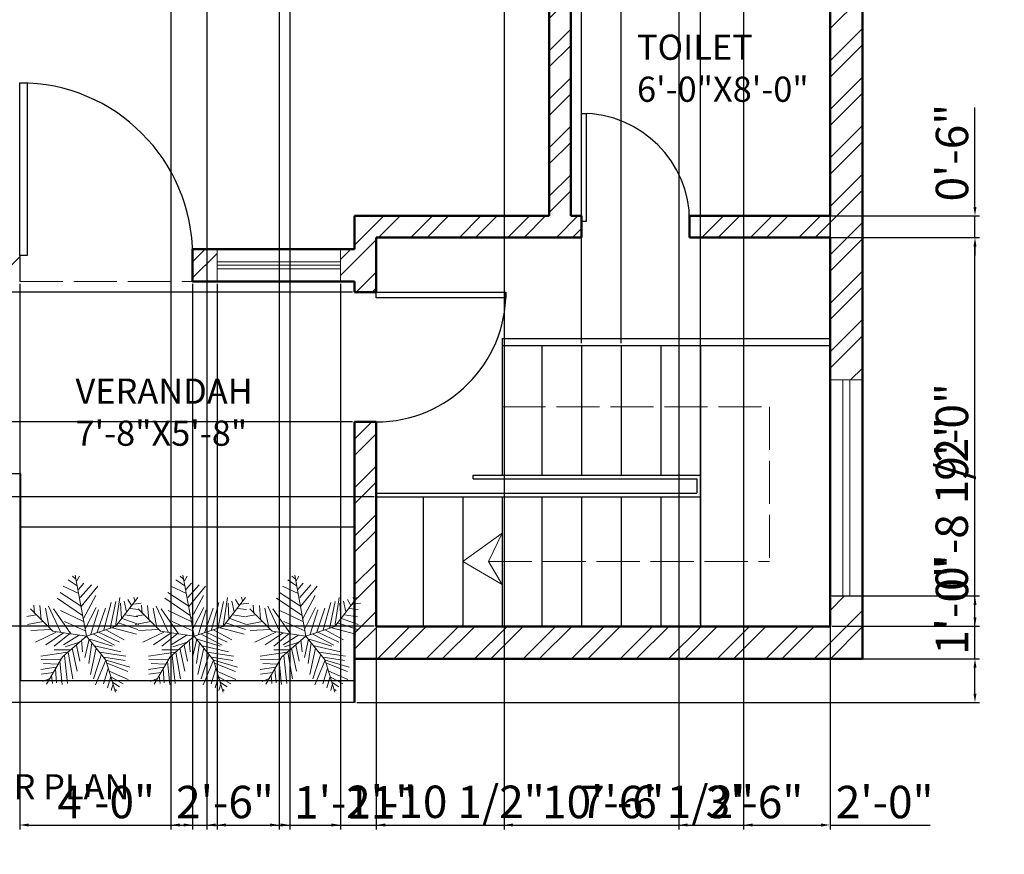
# Model space of a CAD drawing. Units: inches. Extents: x 1104 to 1745, y 678 to 1361.
# Tile 2 of 4: x 1387 to 1660, y 678 to 910. Entities that reach past the tile are written whole.
import ezdxf

# ---------------------------------------------------------------- set-up
doc = ezdxf.new("R2010")
doc.units = ezdxf.units.IN
doc.linetypes.add('ACAD_ISO02W100', pattern=[15, 12, -3])
for name, color, linetype, lineweight in [('A-ANNO-DIMS', 2, 'Continuous', 18), ('A-ANNO-PATH', 2, 'ACAD_ISO02W100', 18), ('A-ANNO-SYMB', 2, 'Continuous', 18), ('A-ANNO-TEXT', 7, 'Continuous', 35), ('A-AREA-IDEN', 7, 'Continuous', 25), ('A-DOOR', 4, 'Continuous', 25), ('A-DOOR-HIDN', 4, 'ACAD_ISO02W100', 18), ('A-FLOR-STRS', 7, 'Continuous', 25), ('A-WALL', 7, 'Continuous', 50), ('A-WALL-PATT', 252, 'ACAD_ISO02W100', 13), ('C-SITE', 8, 'Continuous', 25), ('L-PLNT', 94, 'Continuous', 18)]:
    doc.layers.add(name, color=color, linetype=linetype, lineweight=lineweight)
doc.layers.add('A-GLAZ', color=244, linetype='Continuous', lineweight=18, true_color=0x991b1e)
doc.styles.get("Standard").update_dxf_attribs({"font": 'arial.ttf'})
doc.dimstyles.new('ISO-25', dxfattribs={"dimtxt": 9, "dimasz": 2.5, "dimexe": 1.25, "dimexo": 0.625, "dimtad": 1, "dimlunit": 3, "dimtxsty": 'Standard', "dimcen": 2.5, "dimadec": 0, "dimazin": 0, "dimtfac": 1, "dimtmove": 0, "dimatfit": 3, "dimfxl": 1, "dimarcsym": 0})

# ---------------------------------------------------------------- blocks, each defined once
blk = doc.blocks.new('*U2')
for p, q in [((0, 0), (0, -6)), ((40, 0), (40, -6))]:
    blk.add_line(p, q)
blk.add_lwpolyline([(0, 0), (0, 40), (1.75, 40), (1.75, 0)], close=True)
blk.add_arc((0, 0), 40, 0, 90)
blk = doc.blocks.new('*U5')
for p, q in [((0, 0), (0, -6)), ((40, 0), (40, -6))]:
    blk.add_line(p, q)
blk.add_lwpolyline([(0, 0), (0, 40), (1.75, 40), (1.75, 0)], close=True)
blk.add_arc((0, 0), 40, 0, 90)
blk = doc.blocks.new('*U6')
for p, q in [((-40, 0), (-40, 6)), ((0, 0), (0, 6))]:
    blk.add_line(p, q)
blk.add_lwpolyline([(0, 0), (0, -40), (-1.75, -40), (-1.75, 0)], close=True)
blk.add_arc((0, 0), 40, 180, 270)
blk = doc.blocks.new('*U12')
for p, q in [((-10.186, 53.64), (-13.084, 55.962)), ((0, 0), (-10.5, 57)), ((-9.099, 51.782), (-6.563, 55.962)), ((-7.288, 39.707), (-21.778, 46.673)), ((-8.737, 47.138), (-17.069, 52.711)), ((-7.65, 43.423), (-2.578, 49.46)), ((-5.839, 35.992), (4.667, 48.067)), ((-5.114, 27.632), (10.463, 46.673)), ((-5.114, 28.097), (-24.676, 40.636)), ((-2.941, 16.486), (8.652, 37.85)), ((-48.585, 21.131), (-49.309, 29.026)), ((-43.513, 28.561), (-42.427, 15.558)), ((-35.544, 28.097), (-24.314, 3.947)), ((-3.665, 19.273), (-27.574, 35.527)), ((16.259, 5.805), (23.142, 31.348)), ((22.055, 7.198), (27.489, 32.277)), ((27, 9), (48, 36)), ((27.127, 9.056), (31.112, 35.992)), ((31.836, 30.883), (32.561, 16.486)), ((35.096, 32.741), (37.27, 22.524)), ((38.719, 34.134), (41.979, 28.561)), ((43.791, 29.954), (51.036, 30.883)), ((44.153, 36.456), (45.239, 32.741)), ((-47.498, 19.737), (-55.83, 18.344)), ((-31.5, 4.5), (-52.5, 25.5)), ((-38.442, 26.239), (-34.819, 7.663)), ((-14.533, 2.09), (-30.834, 25.31)), ((-24.314, 23.917), (-2.941, 13.7)), ((-1.129, 6.734), (9.014, 26.704)), ((3.942, 1.625), (11.187, 24.381)), ((10.101, 3.483), (17.708, 26.239)), ((36.183, 19.737), (48.137, 17.88)), ((40.53, 25.775), (48.862, 24.846)), ((-40.615, 13.7), (-55.105, 10.913)), ((-20.691, 13.7), (-1.129, 4.876)), ((29.662, 12.307), (48.137, 6.269)), ((33.285, 16.486), (48.862, 10.913)), ((-33.37, 6.269), (-52.207, 5.34)), ((-28.299, 3.483), (-47.86, -5.805)), ((-21.416, 3.018), (-38.079, -8.128)), ((0, 0), (-31.5, 4.5)), ((-15.982, 2.09), (-30.11, -9.521)), ((0, 0), (-22.5, -19.5)), ((-6.563, 1.161), (-21.416, -8.128)), ((0, 0), (27, 9)), ((0, 0), (18, -22.5)), ((6.478, 1.625), (26.04, -8.592)), ((11.187, 3.483), (30.749, -5.805)), ((18.07, 5.805), (35.096, -3.483)), ((24.229, 7.663), (46.688, 1.625)), ((-6.563, -5.805), (-19.967, -9.985)), ((-9.461, -8.592), (-6.201, -23.453)), ((-4.752, -3.483), (-3.665, -14.629)), ((2.493, -3.019), (-1.491, -20.202)), ((1.769, -2.555), (24.229, -9.521)), ((5.029, -6.27), (2.131, -25.775)), ((7.565, -9.056), (32.198, -14.629)), ((-17.431, -15.094), (-42.789, -18.809)), ((-15.257, -12.772), (-30.11, -12.772)), ((-20.691, -18.345), (-17.793, -44.352)), ((-17.069, -15.094), (-12.721, -40.172)), ((-13.446, -11.378), (-8.737, -32.741)), ((9.014, -11.378), (3.58, -35.992)), ((14.085, -16.951), (6.478, -40.172)), ((12.274, -15.094), (36.907, -18.809)), ((-24.314, -21.596), (-42.427, -22.06)), ((-26.849, -26.24), (-40.253, -25.775)), ((-22.5, -19.5), (-37.5, -45)), ((-25.038, -23.918), (-22.865, -45.281)), ((18.07, -22.524), (8.289, -45.745)), ((16.259, -19.738), (36.183, -22.989)), ((18, -22.5), (27, -52.5)), ((18.433, -22.524), (40.53, -29.026)), ((19.157, -25.311), (38.719, -33.206)), ((-28.299, -29.026), (-42.789, -31.348)), ((-30.834, -34.135), (-42.427, -35.528)), ((-29.023, -30.884), (-27.936, -43.887)), ((20.244, -30.419), (15.897, -44.816)), ((21.331, -32.741), (39.081, -40.636)), ((-34.457, -39.708), (-40.978, -42.494)), ((-32.646, -36.921), (-31.921, -44.352)), ((22.78, -37.85), (19.519, -48.532)), ((22.78, -38.314), (34.372, -44.816)), ((24.591, -45.745), (23.142, -50.854)), ((24.591, -43.423), (30.749, -47.603)), ((26.764, -49.925), (28.213, -50.854))]:
    blk.add_line(p, q)
blk = doc.blocks.new('WIN-GLASS-60IN')
for p, q in [((0, 2), (60, 2)), ((0, 0), (60, 0))]:
    blk.add_line(p, q)
blk = doc.blocks.new('*D33')
at = {"layer": 'A-ANNO-DIMS', "color": 0, "lineweight": -2, "transparency": 16777216}
for p, q in [((1486.11, 740.5), (1486.11, 684.69)), ((1612.11, 740.5), (1612.11, 684.69)), ((1488.61, 685.94), (1609.61, 685.94))]:
    blk.add_line(p, q, dxfattribs=at)
at = {"layer": 'A-ANNO-DIMS', "color": 0, "transparency": 16777216}
for points in [[(1488.61, 686.36), (1488.61, 685.52), (1486.11, 685.94)], [(1609.61, 686.36), (1609.61, 685.52), (1612.11, 685.94)]]:
    blk.add_solid(points, dxfattribs=at)
at = {"layer": 'Defpoints', "color": 0, "transparency": 16777216}
for p in [(1486.11, 741.13), (1612.11, 741.13), (1612.11, 685.94)]:
    blk.add_point(p, dxfattribs=at)
at = {"layer": 'A-ANNO-DIMS', "color": 0, "transparency": 16777216, "insert": (1549.11, 691.16), "char_height": 9, "attachment_point": 5}
blk.add_mtext('10\'-6"', dxfattribs=at)
blk = doc.blocks.new('*D34')
at = {"layer": 'A-ANNO-DIMS', "color": 0, "lineweight": -2, "transparency": 16777216}
for p, q in [((1612.73, 849.13), (1653.59, 849.13)), ((1652.34, 743.63), (1652.34, 846.63)), ((1612.73, 741.13), (1653.59, 741.13))]:
    blk.add_line(p, q, dxfattribs=at)
at = {"layer": 'A-ANNO-DIMS', "color": 0, "transparency": 16777216}
for points in [[(1651.93, 846.63), (1652.76, 846.63), (1652.34, 849.13)], [(1651.93, 743.63), (1652.76, 743.63), (1652.34, 741.13)]]:
    blk.add_solid(points, dxfattribs=at)
at = {"layer": 'Defpoints', "color": 0, "transparency": 16777216}
for p in [(1612.11, 849.13), (1652.34, 849.13), (1612.11, 741.13)]:
    blk.add_point(p, dxfattribs=at)
at = {"layer": 'A-ANNO-DIMS', "color": 0, "transparency": 16777216, "insert": (1647.12, 795.13), "char_height": 9, "attachment_point": 5, "rotation": 90}
blk.add_mtext('9\'-0"', dxfattribs=at)
blk = doc.blocks.new('*D36')
at = {"layer": 'A-ANNO-DIMS', "color": 0, "lineweight": -2, "transparency": 16777216}
for p, q in [((1652.34, 857.63), (1652.34, 885.3)), ((1573.73, 855.13), (1653.59, 855.13)), ((1652.34, 849.13), (1652.34, 855.13)), ((1573.73, 849.13), (1653.59, 849.13)), ((1652.34, 846.63), (1652.34, 844.13))]:
    blk.add_line(p, q, dxfattribs=at)
at = {"layer": 'A-ANNO-DIMS', "color": 0, "transparency": 16777216}
for points in [[(1651.93, 857.63), (1652.76, 857.63), (1652.34, 855.13)], [(1651.93, 846.63), (1652.76, 846.63), (1652.34, 849.13)]]:
    blk.add_solid(points, dxfattribs=at)
at = {"layer": 'Defpoints', "color": 0, "transparency": 16777216}
for p in [(1573.11, 855.13), (1652.34, 855.13), (1573.11, 849.13)]:
    blk.add_point(p, dxfattribs=at)
at = {"layer": 'A-ANNO-DIMS', "color": 0, "transparency": 16777216, "insert": (1647.12, 872.72), "char_height": 9, "attachment_point": 5, "rotation": 90}
blk.add_mtext('0\'-6"', dxfattribs=at)
blk = doc.blocks.new('*D37')
at = {"layer": 'A-ANNO-DIMS', "color": 0, "lineweight": -2, "transparency": 16777216}
for p, q in [((1387.11, 836.3), (1387.11, 684.69)), ((1435.11, 836.3), (1435.11, 684.69)), ((1389.61, 685.94), (1432.61, 685.94))]:
    blk.add_line(p, q, dxfattribs=at)
at = {"layer": 'A-ANNO-DIMS', "color": 0, "transparency": 16777216}
for points in [[(1389.61, 686.36), (1389.61, 685.52), (1387.11, 685.94)], [(1432.61, 686.36), (1432.61, 685.52), (1435.11, 685.94)]]:
    blk.add_solid(points, dxfattribs=at)
at = {"layer": 'Defpoints', "color": 0, "transparency": 16777216}
for p in [(1387.11, 836.92), (1435.11, 836.92), (1435.11, 685.94)]:
    blk.add_point(p, dxfattribs=at)
at = {"layer": 'A-ANNO-DIMS', "color": 0, "transparency": 16777216, "insert": (1411.11, 691.16), "char_height": 9, "attachment_point": 5}
blk.add_mtext('4\'-0"', dxfattribs=at)
blk = doc.blocks.new('*D39')
at = {"layer": 'A-ANNO-DIMS', "color": 0, "lineweight": -2, "transparency": 16777216}
for p, q in [((1429.11, 1148.5), (1429.11, 684.69)), ((1459.11, 1148.5), (1459.11, 684.69)), ((1431.61, 685.94), (1456.61, 685.94))]:
    blk.add_line(p, q, dxfattribs=at)
at = {"layer": 'A-ANNO-DIMS', "color": 0, "transparency": 16777216}
for points in [[(1431.61, 686.36), (1431.61, 685.52), (1429.11, 685.94)], [(1456.61, 686.36), (1456.61, 685.52), (1459.11, 685.94)]]:
    blk.add_solid(points, dxfattribs=at)
at = {"layer": 'Defpoints', "color": 0, "transparency": 16777216}
for p in [(1429.11, 1149.13), (1459.11, 1149.13), (1459.11, 685.94)]:
    blk.add_point(p, dxfattribs=at)
at = {"layer": 'A-ANNO-DIMS', "color": 0, "transparency": 16777216, "insert": (1444.11, 691.16), "char_height": 9, "attachment_point": 5}
blk.add_mtext('2\'-6"', dxfattribs=at)
blk = doc.blocks.new('*D42')
at = {"layer": 'A-ANNO-DIMS', "color": 0, "lineweight": -2, "transparency": 16777216}
for p, q in [((1588.11, 1076.5), (1588.11, 684.69)), ((1612.11, 1076.5), (1612.11, 684.69)), ((1590.61, 685.94), (1609.61, 685.94)), ((1612.11, 685.94), (1639.93, 685.94))]:
    blk.add_line(p, q, dxfattribs=at)
at = {"layer": 'A-ANNO-DIMS', "color": 0, "transparency": 16777216}
for points in [[(1590.61, 686.36), (1590.61, 685.52), (1588.11, 685.94)], [(1609.61, 686.36), (1609.61, 685.52), (1612.11, 685.94)]]:
    blk.add_solid(points, dxfattribs=at)
at = {"layer": 'Defpoints', "color": 0, "transparency": 16777216}
for p in [(1588.11, 1077.13), (1612.11, 1077.13), (1612.11, 685.94)]:
    blk.add_point(p, dxfattribs=at)
at = {"layer": 'A-ANNO-DIMS', "color": 0, "transparency": 16777216, "insert": (1627.27, 691.16), "char_height": 9, "attachment_point": 5}
blk.add_mtext('2\'-0"', dxfattribs=at)
blk = doc.blocks.new('*D43')
at = {"layer": 'A-ANNO-DIMS', "color": 0, "lineweight": -2, "transparency": 16777216}
for p, q in [((1521.6, 956.5), (1521.6, 684.69)), ((1612.11, 956.5), (1612.11, 684.69)), ((1524.1, 685.94), (1609.61, 685.94))]:
    blk.add_line(p, q, dxfattribs=at)
at = {"layer": 'A-ANNO-DIMS', "color": 0, "transparency": 16777216}
for points in [[(1524.1, 686.36), (1524.1, 685.52), (1521.6, 685.94)], [(1609.61, 686.36), (1609.61, 685.52), (1612.11, 685.94)]]:
    blk.add_solid(points, dxfattribs=at)
at = {"layer": 'Defpoints', "color": 0, "transparency": 16777216}
for p in [(1521.6, 957.13), (1612.11, 957.13), (1612.11, 685.94)]:
    blk.add_point(p, dxfattribs=at)
at = {"layer": 'A-ANNO-DIMS', "color": 0, "transparency": 16777216, "insert": (1566.85, 691.22), "char_height": 9, "attachment_point": 5}
blk.add_mtext('7\'-6 1/2"', dxfattribs=at)
blk = doc.blocks.new('*D45')
at = {"layer": 'A-ANNO-DIMS', "color": 0, "lineweight": -2, "transparency": 16777216}
for p, q in [((1652.34, 732.13), (1652.34, 758.96)), ((1480.73, 732.13), (1653.59, 732.13)), ((1652.34, 722.45), (1652.34, 729.63)), ((1480.73, 719.95), (1653.59, 719.95))]:
    blk.add_line(p, q, dxfattribs=at)
at = {"layer": 'A-ANNO-DIMS', "color": 0, "transparency": 16777216}
for points in [[(1651.93, 729.63), (1652.76, 729.63), (1652.34, 732.13)], [(1651.93, 722.45), (1652.76, 722.45), (1652.34, 719.95)]]:
    blk.add_solid(points, dxfattribs=at)
at = {"layer": 'Defpoints', "color": 0, "transparency": 16777216}
for p in [(1480.11, 732.13), (1652.34, 732.13), (1480.11, 719.95)]:
    blk.add_point(p, dxfattribs=at)
at = {"layer": 'A-ANNO-DIMS', "color": 0, "transparency": 16777216, "insert": (1647.12, 746.79), "char_height": 9, "attachment_point": 5, "rotation": 90}
blk.add_mtext('1\'-0"', dxfattribs=at)
blk = doc.blocks.new('*D46')
at = {"layer": 'A-ANNO-DIMS', "color": 0, "lineweight": -2, "transparency": 16777216}
for p, q in [((1441.89, 836.3), (1441.89, 684.69)), ((1476.17, 836.3), (1476.17, 684.69)), ((1444.39, 685.94), (1473.67, 685.94)), ((1476.17, 685.94), (1531.96, 685.94))]:
    blk.add_line(p, q, dxfattribs=at)
at = {"layer": 'A-ANNO-DIMS', "color": 0, "transparency": 16777216}
for points in [[(1444.39, 686.36), (1444.39, 685.52), (1441.89, 685.94)], [(1473.67, 686.36), (1473.67, 685.52), (1476.17, 685.94)]]:
    blk.add_solid(points, dxfattribs=at)
at = {"layer": 'Defpoints', "color": 0, "transparency": 16777216}
for p in [(1441.89, 836.92), (1476.17, 836.92), (1476.17, 685.94)]:
    blk.add_point(p, dxfattribs=at)
at = {"layer": 'A-ANNO-DIMS', "color": 0, "transparency": 16777216, "insert": (1505.31, 691.22), "char_height": 9, "attachment_point": 5}
blk.add_mtext('2\'-10 1/2"', dxfattribs=at)
blk = doc.blocks.new('*D47')
at = {"layer": 'A-ANNO-DIMS', "color": 0, "lineweight": -2, "transparency": 16777216}
for p, q in [((1479.48, 833.92), (1198.71, 833.92)), ((1199.96, 800.42), (1199.96, 831.42)), ((1479.48, 797.92), (1198.71, 797.92))]:
    blk.add_line(p, q, dxfattribs=at)
at = {"layer": 'A-ANNO-DIMS', "color": 0, "transparency": 16777216}
for points in [[(1199.54, 831.42), (1200.37, 831.42), (1199.96, 833.92)], [(1199.54, 800.42), (1200.37, 800.42), (1199.96, 797.92)]]:
    blk.add_solid(points, dxfattribs=at)
at = {"layer": 'Defpoints', "color": 0, "transparency": 16777216}
for p in [(1199.96, 833.92), (1480.11, 833.92), (1480.11, 797.92)]:
    blk.add_point(p, dxfattribs=at)
at = {"layer": 'A-ANNO-DIMS', "color": 0, "transparency": 16777216, "insert": (1194.73, 815.92), "char_height": 9, "attachment_point": 5, "rotation": 90}
blk.add_mtext('3\'-0"', dxfattribs=at)
blk = doc.blocks.new('*D51')
at = {"layer": 'A-ANNO-DIMS', "color": 0, "lineweight": -2, "transparency": 16777216}
for p, q in [((1652.34, 749.56), (1652.34, 798.21)), ((1612.73, 749.56), (1653.59, 749.56)), ((1652.34, 743.63), (1652.34, 747.06)), ((1612.73, 741.13), (1653.59, 741.13))]:
    blk.add_line(p, q, dxfattribs=at)
at = {"layer": 'A-ANNO-DIMS', "color": 0, "transparency": 16777216}
for points in [[(1651.93, 747.06), (1652.76, 747.06), (1652.34, 749.56)], [(1651.93, 743.63), (1652.76, 743.63), (1652.34, 741.13)]]:
    blk.add_solid(points, dxfattribs=at)
at = {"layer": 'Defpoints', "color": 0, "transparency": 16777216}
for p in [(1612.11, 749.56), (1652.34, 749.56), (1612.11, 741.13)]:
    blk.add_point(p, dxfattribs=at)
at = {"layer": 'A-ANNO-DIMS', "color": 0, "transparency": 16777216, "insert": (1647.06, 775.13), "char_height": 9, "attachment_point": 5, "rotation": 90}
blk.add_mtext('0\'-8 1/2"', dxfattribs=at)
blk = doc.blocks.new('*D53')
at = {"layer": 'A-ANNO-DIMS', "color": 0, "lineweight": -2, "transparency": 16777216}
for p, q in [((1576.11, 741.75), (1576.11, 1343.53)), ((1612.11, 741.75), (1612.11, 1343.53)), ((1578.61, 1342.28), (1609.61, 1342.28))]:
    blk.add_line(p, q, dxfattribs=at)
at = {"layer": 'A-ANNO-DIMS', "color": 0, "transparency": 16777216}
for points in [[(1578.61, 1342.7), (1578.61, 1341.86), (1576.11, 1342.28)], [(1609.61, 1342.7), (1609.61, 1341.86), (1612.11, 1342.28)]]:
    blk.add_solid(points, dxfattribs=at)
at = {"layer": 'Defpoints', "color": 0, "transparency": 16777216}
for p in [(1612.11, 1342.28), (1576.11, 741.13), (1612.11, 741.13)]:
    blk.add_point(p, dxfattribs=at)
at = {"layer": 'A-ANNO-DIMS', "color": 0, "transparency": 16777216, "insert": (1594.11, 1347.5), "char_height": 9, "attachment_point": 5}
blk.add_mtext('3\'-0"', dxfattribs=at)
blk = doc.blocks.new('*D54')
at = {"layer": 'A-ANNO-DIMS', "color": 0, "lineweight": -2, "transparency": 16777216}
for p, q in [((1485.48, 777.13), (1198.71, 777.13)), ((1199.96, 743.63), (1199.96, 774.63)), ((1485.48, 741.13), (1198.71, 741.13))]:
    blk.add_line(p, q, dxfattribs=at)
at = {"layer": 'A-ANNO-DIMS', "color": 0, "transparency": 16777216}
for points in [[(1199.54, 774.63), (1200.37, 774.63), (1199.96, 777.13)], [(1199.54, 743.63), (1200.37, 743.63), (1199.96, 741.13)]]:
    blk.add_solid(points, dxfattribs=at)
at = {"layer": 'Defpoints', "color": 0, "transparency": 16777216}
for p in [(1199.96, 777.13), (1486.11, 777.13), (1486.11, 741.13)]:
    blk.add_point(p, dxfattribs=at)
at = {"layer": 'A-ANNO-DIMS', "color": 0, "transparency": 16777216, "insert": (1194.73, 759.13), "char_height": 9, "attachment_point": 5, "rotation": 90}
blk.add_mtext('3\'-0"', dxfattribs=at)
blk = doc.blocks.new('*D55')
at = {"layer": 'A-ANNO-DIMS', "color": 0, "lineweight": -2, "transparency": 16777216}
for p, q in [((1543.11, 819.75), (1543.11, 1343.53)), ((1554.11, 819.75), (1554.11, 1343.53)), ((1545.61, 1342.28), (1551.61, 1342.28)), ((1554.11, 1342.28), (1588.77, 1342.28))]:
    blk.add_line(p, q, dxfattribs=at)
at = {"layer": 'A-ANNO-DIMS', "color": 0, "transparency": 16777216}
for points in [[(1545.61, 1342.7), (1545.61, 1341.86), (1543.11, 1342.28)], [(1551.61, 1342.7), (1551.61, 1341.86), (1554.11, 1342.28)]]:
    blk.add_solid(points, dxfattribs=at)
at = {"layer": 'Defpoints', "color": 0, "transparency": 16777216}
for p in [(1554.11, 1342.28), (1543.11, 819.13), (1554.11, 819.13)]:
    blk.add_point(p, dxfattribs=at)
at = {"layer": 'A-ANNO-DIMS', "color": 0, "transparency": 16777216, "insert": (1572.69, 1347.5), "char_height": 9, "attachment_point": 5}
blk.add_mtext('0\'-11"', dxfattribs=at)
blk = doc.blocks.new('*D57')
at = {"layer": 'A-ANNO-DIMS', "color": 0, "lineweight": -2, "transparency": 16777216}
for p, q in [((1439.05, 1250.5), (1439.05, 684.69)), ((1462.11, 1250.5), (1462.11, 684.69)), ((1441.55, 685.94), (1459.61, 685.94)), ((1462.11, 685.94), (1495.93, 685.94))]:
    blk.add_line(p, q, dxfattribs=at)
at = {"layer": 'A-ANNO-DIMS', "color": 0, "transparency": 16777216}
for points in [[(1441.55, 686.36), (1441.55, 685.52), (1439.05, 685.94)], [(1459.61, 686.36), (1459.61, 685.52), (1462.11, 685.94)]]:
    blk.add_solid(points, dxfattribs=at)
at = {"layer": 'Defpoints', "color": 0, "transparency": 16777216}
for p in [(1439.05, 1251.13), (1462.11, 1251.13), (1462.11, 685.94)]:
    blk.add_point(p, dxfattribs=at)
at = {"layer": 'A-ANNO-DIMS', "color": 0, "transparency": 16777216, "insert": (1480.27, 691.08), "char_height": 9, "attachment_point": 5}
blk.add_mtext('1\'-11"', dxfattribs=at)
blk = doc.blocks.new('*D58')
at = {"layer": 'A-ANNO-DIMS', "color": 0, "lineweight": -2, "transparency": 16777216}
for p, q in [((1570.11, 1250.5), (1570.11, 684.69)), ((1612.11, 1250.5), (1612.11, 684.69)), ((1572.61, 685.94), (1609.61, 685.94))]:
    blk.add_line(p, q, dxfattribs=at)
at = {"layer": 'A-ANNO-DIMS', "color": 0, "transparency": 16777216}
for points in [[(1572.61, 686.36), (1572.61, 685.52), (1570.11, 685.94)], [(1609.61, 686.36), (1609.61, 685.52), (1612.11, 685.94)]]:
    blk.add_solid(points, dxfattribs=at)
at = {"layer": 'Defpoints', "color": 0, "transparency": 16777216}
for p in [(1570.11, 1251.13), (1612.11, 1251.13), (1612.11, 685.94)]:
    blk.add_point(p, dxfattribs=at)
at = {"layer": 'A-ANNO-DIMS', "color": 0, "transparency": 16777216, "insert": (1591.11, 691.16), "char_height": 9, "attachment_point": 5}
blk.add_mtext('3\'-6"', dxfattribs=at)

msp = doc.modelspace()

# ---------------------------------------------------------------- hatches: boundary and pattern name
at = {"layer": 'A-WALL-PATT'}
h = msp.add_hatch(dxfattribs=at)
h.set_pattern_fill('ANSI32', color=256)
h.paths.add_polyline_path([(1277.606, 917.921), (1240.106, 917.921), (1240.106, 980.462), (1231.106, 980.462), (1231.106, 719.949), (1240.106, 719.949), (1240.106, 908.921), (1277.606, 908.921)])
h.paths.add_polyline_path([(1384.106, 917.921), (1337.606, 917.921), (1337.606, 908.921), (1375.106, 908.921), (1375.106, 836.921), (1387.106, 836.921), (1387.106, 844.121), (1387.106, 845.921), (1384.106, 845.921)])
h.paths.add_polyline_path([(1486.106, 849.129), (1543.106, 849.129), (1543.106, 855.129), (1540.106, 855.129), (1540.106, 951.129), (1612.106, 951.129), (1612.106, 941.864), (1621.106, 941.864), (1621.106, 986.665), (1612.106, 986.665), (1612.106, 957.129), (1486.106, 957.129), (1486.106, 1017.129), (1480.106, 1017.129), (1480.106, 951.129), (1534.106, 951.129), (1534.106, 855.129), (1480.106, 855.129), (1480.106, 845.921), (1476.166, 845.921), (1476.166, 836.921), (1480.106, 836.921), (1480.106, 833.921), (1486.106, 833.921)])
h.paths.add_polyline_path([(1441.89, 845.921), (1435.106, 845.921), (1435.106, 836.921), (1441.89, 836.921)])
h.paths.add_polyline_path([(1240.106, 1137.841), (1231.106, 1137.841), (1231.106, 1040.462), (1240.106, 1040.462), (1240.106, 1077.129), (1390.106, 1077.129), (1390.106, 1086.129), (1384.106, 1086.129), (1384.106, 1083.129), (1240.106, 1083.129)])
h.paths.add_polyline_path([(1621.106, 1146.091), (1612.106, 1146.091), (1612.106, 1083.129), (1468.106, 1083.129), (1468.106, 1086.129), (1462.106, 1086.129), (1462.106, 1077.129), (1480.106, 1077.129), (1612.106, 1077.129), (1612.106, 1046.665), (1621.106, 1046.665)])
h.paths.add_polyline_path([(1240.106, 1251.129), (1282.106, 1251.129), (1282.106, 1260.129), (1231.106, 1260.129), (1231.106, 1197.841), (1240.106, 1197.841)])
h.paths.add_polyline_path([(1418.05, 1260.129), (1342.106, 1260.129), (1342.106, 1251.129), (1384.106, 1251.129), (1384.106, 1122.129), (1390.106, 1122.129), (1390.106, 1149.129), (1429.106, 1149.129), (1429.106, 1155.129), (1390.106, 1155.129), (1390.106, 1251.129), (1418.05, 1251.129)])
h.paths.add_polyline_path([(1510.106, 1260.129), (1439.05, 1260.129), (1439.05, 1251.129), (1462.106, 1251.129), (1462.106, 1155.129), (1459.106, 1155.129), (1459.106, 1153.629), (1459.106, 1149.129), (1462.106, 1149.129), (1462.106, 1122.129), (1468.106, 1122.129), (1468.106, 1251.129), (1510.106, 1251.129)])
h.paths.add_polyline_path([(1621.106, 1260.129), (1570.106, 1260.129), (1570.106, 1251.129), (1612.106, 1251.129), (1612.106, 1206.091), (1621.106, 1206.091)])
h.paths.add_polyline_path([(1621.106, 920.864), (1612.106, 920.864), (1612.106, 855.129), (1573.106, 855.129), (1573.106, 849.129), (1612.106, 849.129), (1612.106, 809.56), (1621.106, 809.56)])
h.paths.add_polyline_path([(1621.106, 749.56), (1612.106, 749.56), (1612.106, 741.129), (1486.106, 741.129), (1486.106, 797.921), (1480.106, 797.921), (1480.106, 732.129), (1621.106, 732.129)])

# ---------------------------------------------------------------- linework, layer by layer
at = {"layer": 'A-ANNO-PATH'}
for p, q in [((1521.106, 802.129), (1595.31, 802.129)), ((1595.31, 802.129), (1595.31, 759.129)), ((1517.274, 759.129), (1595.31, 759.129))]:
    msp.add_line(p, q, dxfattribs=at)
at = {"layer": 'A-ANNO-SYMB'}
for p, q in [((1510.106, 759.129), (1521.106, 766.994)), ((1521.106, 766.994), (1517.274, 759.129)), ((1521.106, 752.741), (1510.106, 759.129)), ((1517.274, 759.129), (1521.106, 752.741))]:
    msp.add_line(p, q, dxfattribs=at)
at = {"layer": 'A-DOOR-HIDN'}
msp.add_line((1387.106, 836.921), (1435.106, 836.921), dxfattribs=at)
at = {"layer": 'A-FLOR-STRS'}
for p, q in [((1521.106, 821.129), (1612.106, 821.129)), ((1521.106, 821.129), (1521.106, 783.129)), ((1521.106, 819.129), (1612.106, 819.129)), ((1532.106, 819.129), (1532.106, 783.129)), ((1543.106, 819.129), (1543.106, 783.129)), ((1554.106, 819.129), (1554.106, 783.129)), ((1565.106, 819.129), (1565.106, 783.129)), ((1576.106, 819.129), (1576.106, 741.129)), ((1512.984, 783.129), (1576.106, 783.129)), ((1512.984, 782.129), (1512.984, 783.129)), ((1512.984, 782.129), (1575.106, 782.129)), ((1575.106, 782.129), (1575.106, 778.129)), ((1486.106, 778.129), (1575.106, 778.129)), ((1486.106, 777.129), (1576.106, 777.129)), ((1499.106, 777.129), (1499.106, 741.129)), ((1510.106, 777.129), (1510.106, 741.129)), ((1521.106, 777.129), (1521.106, 741.129)), ((1532.106, 777.129), (1532.106, 741.129)), ((1543.106, 777.129), (1543.106, 741.129)), ((1554.106, 777.129), (1554.106, 741.129)), ((1565.106, 777.129), (1565.106, 741.129))]:
    msp.add_line(p, q, dxfattribs=at)
at = {"layer": 'A-GLAZ'}
for p, q in [((1441.89, 842.421), (1476.166, 842.421)), ((1441.89, 841.421), (1476.166, 841.421)), ((1441.89, 840.421), (1476.166, 840.421))]:
    msp.add_line(p, q, dxfattribs=at)
for points in [[(1441.89, 845.921), (1476.166, 845.921), (1476.166, 836.921), (1441.89, 836.921)], [(1621.106, 809.56), (1621.106, 749.56), (1612.106, 749.56), (1612.106, 809.56)]]:
    msp.add_lwpolyline(points, close=True, dxfattribs=at)
at = {"layer": 'A-WALL'}
for p, q in [((1621.106, 1260.129), (1621.106, 732.129)), ((1534.106, 951.129), (1534.106, 855.129)), ((1540.106, 951.129), (1540.106, 855.129)), ((1612.106, 951.129), (1612.106, 855.129)), ((1480.106, 855.129), (1534.106, 855.129)), ((1480.106, 855.129), (1480.106, 845.921)), ((1540.106, 855.129), (1543.106, 855.129)), ((1543.106, 855.129), (1543.106, 849.129)), ((1573.106, 855.129), (1573.106, 849.129)), ((1573.106, 855.129), (1612.106, 855.129)), ((1486.106, 849.129), (1486.106, 833.921)), ((1486.106, 849.129), (1543.106, 849.129)), ((1573.106, 849.129), (1612.106, 849.129)), ((1612.106, 849.129), (1612.106, 741.129)), ((1435.106, 845.921), (1435.106, 836.921)), ((1435.106, 845.921), (1480.106, 845.921)), ((1435.106, 836.921), (1480.106, 836.921)), ((1480.106, 836.921), (1480.106, 833.921)), ((1480.106, 833.921), (1486.106, 833.921)), ((1480.106, 797.921), (1486.106, 797.921)), ((1480.106, 797.921), (1480.106, 719.949)), ((1486.106, 797.921), (1486.106, 741.129)), ((1486.106, 741.129), (1612.106, 741.129)), ((1480.106, 732.129), (1621.106, 732.129))]:
    msp.add_line(p, q, dxfattribs=at)
at = {"layer": 'C-SITE'}
for p, q in [((1387.451, 783.475), (1375.451, 783.475)), ((1387.451, 725.949), (1387.451, 783.475)), ((1480.106, 768.707), (1387.451, 768.707)), ((1486.106, 732.129), (1486.106, 731.949)), ((1480.106, 725.949), (1387.451, 725.949)), ((1480.106, 719.949), (1231.106, 719.949))]:
    msp.add_line(p, q, dxfattribs=at)

# ---------------------------------------------------------------- block references
at = {"layer": 'A-DOOR'}
for name, p, xscale, yscale, zscale in [('*U2', (1387.106, 844.121), 1.200000000000001, 1.200000000000001, 1.200000000000001), ('*U5', (1543.106, 853.629), 0.7499999999999887, 0.7499999999999887, 0.7499999999999887)]:
    msp.add_blockref(name, p, dxfattribs=dict(at, xscale=xscale, yscale=yscale, zscale=zscale))
at = {"layer": 'A-DOOR', "xscale": 0.9000000000000049, "yscale": 0.9000000000000049, "zscale": 0.9000000000000049, "rotation": 90}
msp.add_blockref('*U6', (1486.106, 833.921), dxfattribs=at)
at = {"layer": 'A-GLAZ', "rotation": 269.9999999999992}
msp.add_blockref('WIN-GLASS-60IN', (1615.607, 809.561), dxfattribs=at)
at = {"layer": 'L-PLNT', "xscale": 0.2968663969365763, "yscale": 0.2968663969365763, "zscale": 0.2968663969365763}
for p in [(1405.662, 738.432), (1435.548, 738.432), (1466.582, 738.432)]:
    msp.add_blockref('*U12', p, dxfattribs=at)

# ---------------------------------------------------------------- texts
at = {"layer": 'A-ANNO-TEXT', "insert": (1318.552, 700.062), "char_height": 7, "attachment_point": 1}
msp.add_mtext_dynamic_manual_height_columns('GROUND FLOOR PLAN', width=110.84972, gutter_width=12.5, heights=[0], dxfattribs=at)
at = {"layer": 'A-AREA-IDEN', "char_height": 7, "attachment_point": 1}
for s, width, insert in [('TOILET 6\'-0"X8\'-0"', 44.67286, (1558.502, 905.501)), ('VERANDAH\\P7\'-8"X5\'-8"', 55.15613, (1402.602, 809.96))]:
    msp.add_mtext_dynamic_manual_height_columns(s, width=width, gutter_width=12.5, heights=[0], dxfattribs=dict(at, insert=insert))

# ---------------------------------------------------------------- dimensions: what is measured, and where the dimension line sits
at = {"layer": 'A-ANNO-DIMS'}
for base, p1, p2, picture, middle in [((1554.106, 1342.279), (1543.106, 819.129), (1554.106, 819.129), '*D55', (1572.69, 1347.499)), ((1612.106, 1342.279), (1576.106, 741.129), (1612.106, 741.129), '*D53', (1594.106, 1347.502)), ((1462.106, 685.941), (1439.05, 1251.129), (1462.106, 1251.129), '*D57', (1480.266, 691.084)), ((1612.106, 685.941), (1570.106, 1251.129), (1612.106, 1251.129), '*D58', (1591.106, 691.164)), ((1459.106, 685.941), (1429.106, 1149.129), (1459.106, 1149.129), '*D39', (1444.106, 691.161)), ((1612.106, 685.941), (1588.106, 1077.129), (1612.106, 1077.129), '*D42', (1627.27, 691.161)), ((1612.106, 685.941), (1521.602, 957.129), (1612.106, 957.129), '*D43', (1566.854, 691.219)), ((1435.106, 685.941), (1387.106, 836.921), (1435.106, 836.921), '*D37', (1411.106, 691.161)), ((1476.166, 685.941), (1441.89, 836.921), (1476.166, 836.921), '*D46', (1505.312, 691.219)), ((1612.106, 685.941), (1486.106, 741.129), (1612.106, 741.129), '*D33', (1549.106, 691.161))]:
    dim = msp.add_linear_dim(base=base, p1=p1, p2=p2, dimstyle='ISO-25', override={"dimdec": 1, "dimlfac": 1, "dimrnd": 0, "dimzin": 1, "dimdsep": 46, "dimlunit": 4, "dimfrac": 2}, dxfattribs=at)
    dim.commit()
    dim.dimension.update_dxf_attribs({"geometry": picture, "text_midpoint": middle})
for base, p1, p2, picture, middle in [((1652.342, 855.129), (1573.106, 849.129), (1573.106, 855.129), '*D36', (1647.122, 872.716)), ((1652.342, 849.129), (1612.106, 741.129), (1612.106, 849.129), '*D34', (1647.122, 795.129)), ((1199.956, 833.921), (1480.106, 797.921), (1480.106, 833.921), '*D47', (1194.733, 815.921)), ((1652.342, 749.56), (1612.106, 741.129), (1612.106, 749.56), '*D51', (1647.064, 775.133)), ((1199.956, 777.129), (1486.106, 741.129), (1486.106, 777.129), '*D54', (1194.733, 759.129)), ((1652.342, 732.129), (1480.106, 719.949), (1480.106, 732.129), '*D45', (1647.122, 746.792))]:
    dim = msp.add_linear_dim(base=base, p1=p1, p2=p2, angle=90, dimstyle='ISO-25', override={"dimdec": 1, "dimlfac": 1, "dimrnd": 0, "dimzin": 1, "dimdsep": 46, "dimlunit": 4, "dimfrac": 2}, dxfattribs=at)
    dim.commit()
    dim.dimension.update_dxf_attribs({"geometry": picture, "text_midpoint": middle})

doc.saveas('drawing.dxf')
